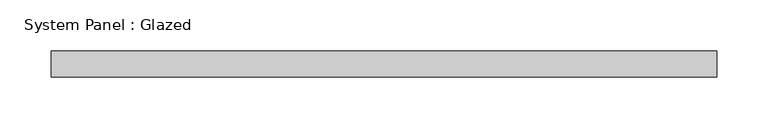
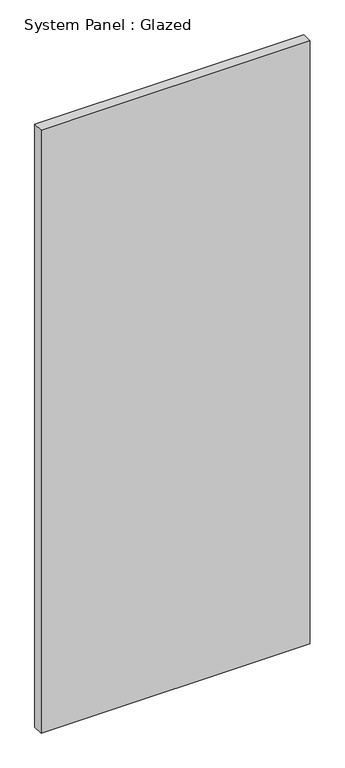
"""IFC4 building model written with IfcOpenShell, lengths in millimetres: plate geometry, System Panel : Glazed."""

from ifc_helpers import new_model, si_unit, origin, origin_with_axes, place, context, project, spatial, polyline, outline, extrude, source, transform, mapped, element, save


def system_panel_glazed_5fa6f1c3(model_context):
    return source(origin(), model_context, "Body", "SweptSolid", [
        extrude(outline(polyline([(323.85, 19.05), (-323.85, 19.05), (-323.85, 44.45), (323.85, 44.45), (323.85, 19.05)])), origin_with_axes(), (0.0, 0.0, 1.0), 1533.012385),
    ])


if __name__ == "__main__":
    model = new_model("IFC4")
    model_context = context("Model", 3, world=origin())
    ifc_project = project(units=[si_unit("LENGTHUNIT", "METRE", prefix="MILLI")], contexts=[model_context])
    site = spatial("IfcSite", under=ifc_project)
    building = spatial("IfcBuilding", under=site)
    placement = place(None, origin())
    system_panel_glazed_shape = system_panel_glazed_5fa6f1c3(model_context)
    element("IfcPlate", 1, ObjectType="System Panel : Glazed", at=placement, inside=building, context=model_context, shape_type="MappedRepresentation", body=[
        mapped(system_panel_glazed_shape, transform((0.0, 0.0, 0.0), x_axis=(1.0, 0.0, 0.0), y_axis=(0.0, 1.0, 0.0), z_axis=(0.0, 0.0, 1.0))),
    ])
    save(model, "model.ifc")

# Revit data of these elements
# Type "System Panel : Glazed"
#   Construction Type Id = "GSP4R"
#   Analytic Construction = "1/8 in Pilkington single glazing"
#   Visual Light Transmittance = 0.9
#   Solar Heat Gain Coefficient = 0.86
#   Heat Transfer Coefficient (U) = 1.18115 BTU/(h·ft²·°F)
#   Define Thermal Properties by = 1
# Element 1 (IfcPlate, "System Panel : Glazed")
#   Materials on its faces: "Glass"
# Materials
#   "Glass": class "Glass", colour RGB 0 128 192, transparency 0.75, Description = "Soda Lime Glass", Cost = 0
